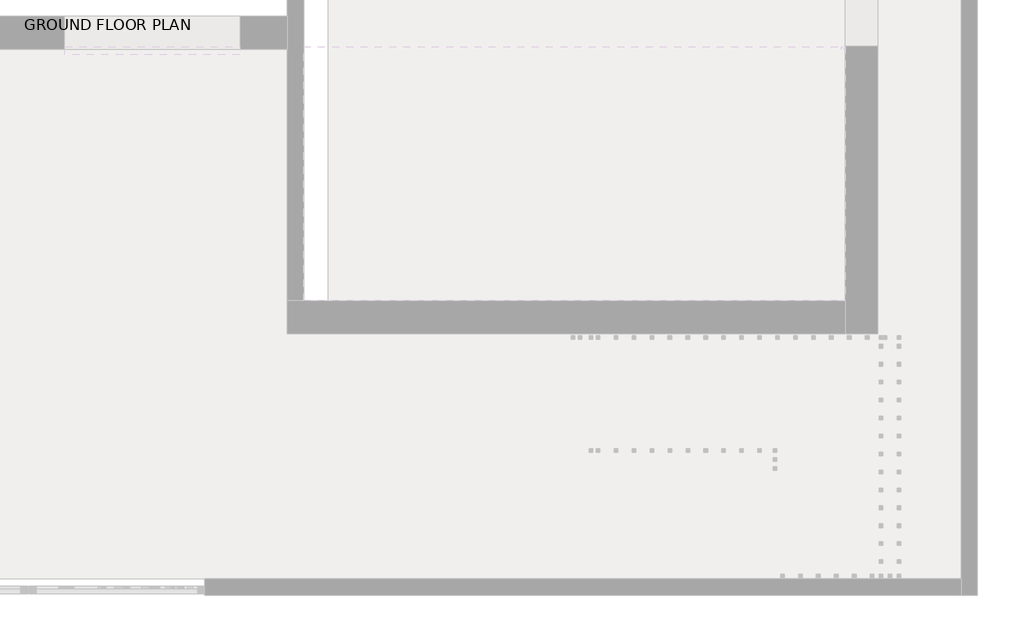
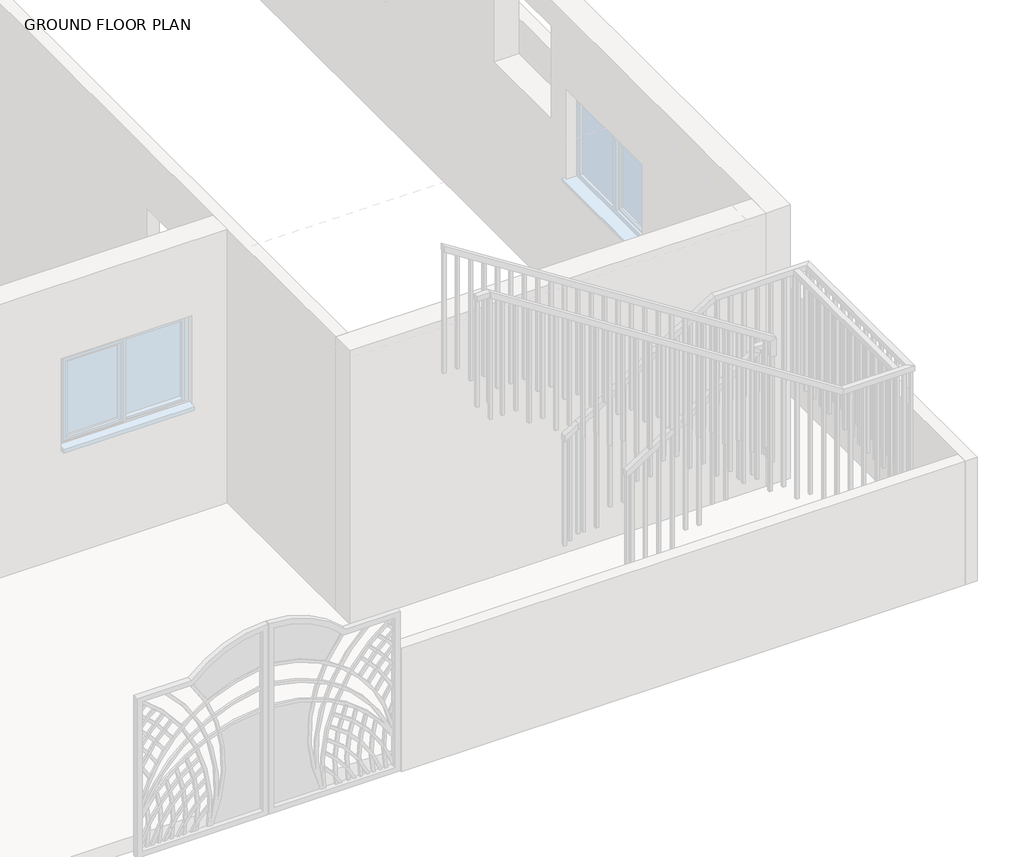
# One storey, part 19 of 23: 2 railings.
"""IFC4 building model written with IfcOpenShell, lengths in millimetres."""

from ifc_helpers import new_model, si_unit, frame, origin, place, context, project, spatial, polyline, outline, extrude, faceted_brep, element, save

model = new_model("IFC4")

# Units and contexts
model_context = context("Model", 3, world=origin())
ifc_project = project(units=[si_unit("LENGTHUNIT", "METRE", prefix="MILLI")], contexts=[model_context])

# Site, building, storey
site = spatial("IfcSite", under=ifc_project)
building = spatial("IfcBuilding", under=site)
storey = spatial("IfcBuildingStorey", under=building, Name="GROUND FLOOR PLAN", Elevation=487.68)

# Railings
placement = place(None, origin())
element("IfcRailing", 1, ObjectType="1100mm", at=placement, inside=storey, context=model_context, shape_type="SolidModel", body=[
    faceted_brep([(-8680.149573, -10220.0521308, 1912.8), (-8680.149573, -10220.0521308, 1853.4423995), (-8680.149573, -10270.0521308, 1853.4423995), (-8680.149573, -10270.0521308, 1912.8), (-7409.7306254, -10220.0521308, 2725.6), (-7395.1045513, -10220.0521308, 2675.6), (-7395.1045513, -10270.0521308, 2675.6), (-7409.7306254, -10270.0521308, 2725.6), (-6495.8132565, -10220.0521308, 2725.6), (-6495.8132565, -10220.0521308, 2675.6), (-6545.8132565, -10270.0521308, 2675.6), (-6545.8132565, -10270.0521308, 2725.6), (-6495.8132565, -11933.6860066, 2725.6), (-6495.8132565, -11933.6860066, 2675.6), (-6545.8132565, -11883.6860066, 2675.6), (-6545.8132565, -11883.6860066, 2725.6), (-7155.718398, -11933.6860066, 2725.6), (-7170.3479429, -11933.6860066, 2675.6), (-7170.3479429, -11883.6860066, 2675.6), (-7155.718398, -11883.6860066, 2725.6), (-10457.8773536, -11933.6860066, 4838.88), (-10457.8773536, -11883.6860066, 4838.88), (-10457.8773536, -11883.6860066, 4779.517542), (-10457.8773536, -11933.6860066, 4779.517542)], [[[0, 1, 2, 3]], [[1, 0, 4, 5]], [[2, 1, 5, 6]], [[3, 2, 6, 7]], [[0, 3, 7, 4]], [[5, 4, 8, 9]], [[6, 5, 9, 10]], [[7, 6, 10, 11]], [[4, 7, 11, 8]], [[9, 8, 12, 13]], [[10, 9, 13, 14]], [[11, 10, 14, 15]], [[8, 11, 15, 12]], [[13, 12, 16, 17]], [[14, 13, 17, 18]], [[15, 14, 18, 19]], [[12, 15, 19, 16]], [[20, 21, 22, 23]], [[17, 16, 20, 23]], [[18, 17, 23, 22]], [[19, 18, 22, 21]], [[16, 19, 21, 20]]]),
    extrude(outline(polyline([(4691.8007425, -10320.8132565), (4707.7999723, -10345.8132565), (3576.32, -10345.8132565), (3576.32, -10320.8132565), (4691.8007425, -10320.8132565)])), frame((0.0, -11921.1860066, 0.0), z_axis=(0.0, 1.0, 0.0), x_axis=(0.0, 0.0, 1.0)), (0.0, 0.0, 1.0), 25.0),
    extrude(outline(polyline([(4611.8045935, -10195.8132565), (4627.8038233, -10220.8132565), (3576.32, -10220.8132565), (3576.32, -10195.8132565), (4611.8045935, -10195.8132565)])), frame((0.0, -11921.1860066, 0.0), z_axis=(0.0, 1.0, 0.0), x_axis=(0.0, 0.0, 1.0)), (0.0, 0.0, 1.0), 25.0),
    extrude(outline(polyline([(4531.8084444, -10070.8132565), (4547.8076742, -10095.8132565), (3413.76, -10095.8132565), (3413.76, -10070.8132565), (4531.8084444, -10070.8132565)])), frame((0.0, -11921.1860066, 0.0), z_axis=(0.0, 1.0, 0.0), x_axis=(0.0, 0.0, 1.0)), (0.0, 0.0, 1.0), 25.0),
    extrude(outline(polyline([(4451.8122954, -9945.8132565), (4467.8115252, -9970.8132565), (3413.76, -9970.8132565), (3413.76, -9945.8132565), (4451.8122954, -9945.8132565)])), frame((0.0, -11921.1860066, 0.0), z_axis=(0.0, 1.0, 0.0), x_axis=(0.0, 0.0, 1.0)), (0.0, 0.0, 1.0), 25.0),
    extrude(outline(polyline([(4371.8161463, -9820.8132565), (4387.8153761, -9845.8132565), (3251.2, -9845.8132565), (3251.2, -9820.8132565), (4371.8161463, -9820.8132565)])), frame((0.0, -11921.1860066, 0.0), z_axis=(0.0, 1.0, 0.0), x_axis=(0.0, 0.0, 1.0)), (0.0, 0.0, 1.0), 25.0),
    extrude(outline(polyline([(4291.8423995, -9695.8132565), (4307.8371231, -9720.8132565), (3251.2, -9720.8132565), (3251.2, -9695.8132565), (4291.8423995, -9695.8132565)])), frame((0.0, -11921.1860066, 0.0), z_axis=(0.0, 1.0, 0.0), x_axis=(0.0, 0.0, 1.0)), (0.0, 0.0, 1.0), 25.0),
    extrude(outline(polyline([(4211.8238482, -9570.8132565), (4227.823078, -9595.8132565), (3088.64, -9595.8132565), (3088.64, -9570.8132565), (4211.8238482, -9570.8132565)])), frame((0.0, -11921.1860066, 0.0), z_axis=(0.0, 1.0, 0.0), x_axis=(0.0, 0.0, 1.0)), (0.0, 0.0, 1.0), 25.0),
    extrude(outline(polyline([(4131.8276992, -9445.8132565), (4147.826929, -9470.8132565), (3088.64, -9470.8132565), (3088.64, -9445.8132565), (4131.8276992, -9445.8132565)])), frame((0.0, -11921.1860066, 0.0), z_axis=(0.0, 1.0, 0.0), x_axis=(0.0, 0.0, 1.0)), (0.0, 0.0, 1.0), 25.0),
    extrude(outline(polyline([(4051.8315501, -9320.8132565), (4067.8307799, -9345.8132565), (2926.08, -9345.8132565), (2926.08, -9320.8132565), (4051.8315501, -9320.8132565)])), frame((0.0, -11921.1860066, 0.0), z_axis=(0.0, 1.0, 0.0), x_axis=(0.0, 0.0, 1.0)), (0.0, 0.0, 1.0), 25.0),
    extrude(outline(polyline([(3971.835401, -9195.8132565), (3987.8346309, -9220.8132565), (2926.08, -9220.8132565), (2926.08, -9195.8132565), (3971.835401, -9195.8132565)])), frame((0.0, -11921.1860066, 0.0), z_axis=(0.0, 1.0, 0.0), x_axis=(0.0, 0.0, 1.0)), (0.0, 0.0, 1.0), 25.0),
    extrude(outline(polyline([(3891.839252, -9070.8132565), (3907.8384818, -9095.8132565), (2763.52, -9095.8132565), (2763.52, -9070.8132565), (3891.839252, -9070.8132565)])), frame((0.0, -11921.1860066, 0.0), z_axis=(0.0, 1.0, 0.0), x_axis=(0.0, 0.0, 1.0)), (0.0, 0.0, 1.0), 25.0),
    extrude(outline(polyline([(3811.8431029, -8945.8132565), (3827.8423328, -8970.8132565), (2763.52, -8970.8132565), (2763.52, -8945.8132565), (3811.8431029, -8945.8132565)])), frame((0.0, -11921.1860066, 0.0), z_axis=(0.0, 1.0, 0.0), x_axis=(0.0, 0.0, 1.0)), (0.0, 0.0, 1.0), 25.0),
    extrude(outline(polyline([(3731.8469539, -8820.8132565), (3747.8461837, -8845.8132565), (2600.96, -8845.8132565), (2600.96, -8820.8132565), (3731.8469539, -8820.8132565)])), frame((0.0, -11921.1860066, 0.0), z_axis=(0.0, 1.0, 0.0), x_axis=(0.0, 0.0, 1.0)), (0.0, 0.0, 1.0), 25.0),
    extrude(outline(polyline([(3651.8508048, -8695.8132565), (3667.8500347, -8720.8132565), (2600.96, -8720.8132565), (2600.96, -8695.8132565), (3651.8508048, -8695.8132565)])), frame((0.0, -11921.1860066, 0.0), z_axis=(0.0, 1.0, 0.0), x_axis=(0.0, 0.0, 1.0)), (0.0, 0.0, 1.0), 25.0),
    extrude(outline(polyline([(3571.8546558, -8570.8132565), (3587.8538856, -8595.8132565), (2438.4, -8595.8132565), (2438.4, -8570.8132565), (3571.8546558, -8570.8132565)])), frame((0.0, -11921.1860066, 0.0), z_axis=(0.0, 1.0, 0.0), x_axis=(0.0, 0.0, 1.0)), (0.0, 0.0, 1.0), 25.0),
    extrude(outline(polyline([(3491.8585067, -8445.8132565), (3507.8577365, -8470.8132565), (2438.4, -8470.8132565), (2438.4, -8445.8132565), (3491.8585067, -8445.8132565)])), frame((0.0, -11921.1860066, 0.0), z_axis=(0.0, 1.0, 0.0), x_axis=(0.0, 0.0, 1.0)), (0.0, 0.0, 1.0), 25.0),
    extrude(outline(polyline([(3411.8623577, -8320.8132565), (3427.8615875, -8345.8132565), (2275.84, -8345.8132565), (2275.84, -8320.8132565), (3411.8623577, -8320.8132565)])), frame((0.0, -11921.1860066, 0.0), z_axis=(0.0, 1.0, 0.0), x_axis=(0.0, 0.0, 1.0)), (0.0, 0.0, 1.0), 25.0),
    extrude(outline(polyline([(3331.8662086, -8195.8132565), (3347.8654384, -8220.8132565), (2275.84, -8220.8132565), (2275.84, -8195.8132565), (3331.8662086, -8195.8132565)])), frame((0.0, -11921.1860066, 0.0), z_axis=(0.0, 1.0, 0.0), x_axis=(0.0, 0.0, 1.0)), (0.0, 0.0, 1.0), 25.0),
    extrude(outline(polyline([(3251.8700596, -8070.8132565), (3267.8692894, -8095.8132565), (2113.28, -8095.8132565), (2113.28, -8070.8132565), (3251.8700596, -8070.8132565)])), frame((0.0, -11921.1860066, 0.0), z_axis=(0.0, 1.0, 0.0), x_axis=(0.0, 0.0, 1.0)), (0.0, 0.0, 1.0), 25.0),
    extrude(outline(polyline([(3171.8739105, -7945.8132565), (3187.8731403, -7970.8132565), (2113.28, -7970.8132565), (2113.28, -7945.8132565), (3171.8739105, -7945.8132565)])), frame((0.0, -11921.1860066, 0.0), z_axis=(0.0, 1.0, 0.0), x_axis=(0.0, 0.0, 1.0)), (0.0, 0.0, 1.0), 25.0),
    extrude(outline(polyline([(3091.8777615, -7820.8132565), (3107.8769913, -7845.8132565), (1950.72, -7845.8132565), (1950.72, -7820.8132565), (3091.8777615, -7820.8132565)])), frame((0.0, -11921.1860066, 0.0), z_axis=(0.0, 1.0, 0.0), x_axis=(0.0, 0.0, 1.0)), (0.0, 0.0, 1.0), 25.0),
    extrude(outline(polyline([(3011.8816124, -7695.8132565), (3027.8808422, -7720.8132565), (1950.72, -7720.8132565), (1950.72, -7695.8132565), (3011.8816124, -7695.8132565)])), frame((0.0, -11921.1860066, 0.0), z_axis=(0.0, 1.0, 0.0), x_axis=(0.0, 0.0, 1.0)), (0.0, 0.0, 1.0), 25.0),
    extrude(outline(polyline([(2931.8854634, -7570.8132565), (2947.8846932, -7595.8132565), (1788.16, -7595.8132565), (1788.16, -7570.8132565), (2931.8854634, -7570.8132565)])), frame((0.0, -11921.1860066, 0.0), z_axis=(0.0, 1.0, 0.0), x_axis=(0.0, 0.0, 1.0)), (0.0, 0.0, 1.0), 25.0),
    extrude(outline(polyline([(2851.8893143, -7445.8132565), (2867.8885441, -7470.8132565), (1788.16, -7470.8132565), (1788.16, -7445.8132565), (2851.8893143, -7445.8132565)])), frame((0.0, -11921.1860066, 0.0), z_axis=(0.0, 1.0, 0.0), x_axis=(0.0, 0.0, 1.0)), (0.0, 0.0, 1.0), 25.0),
    extrude(outline(polyline([(2771.8931653, -7320.8132565), (2787.8923951, -7345.8132565), (1625.6, -7345.8132565), (1625.6, -7320.8132565), (2771.8931653, -7320.8132565)])), frame((0.0, -11921.1860066, 0.0), z_axis=(0.0, 1.0, 0.0), x_axis=(0.0, 0.0, 1.0)), (0.0, 0.0, 1.0), 25.0),
    extrude(outline(polyline([(2691.8970162, -7195.8132565), (2707.896246, -7220.8132565), (1625.6, -7220.8132565), (1625.6, -7195.8132565), (2691.8970162, -7195.8132565)])), frame((0.0, -11921.1860066, 0.0), z_axis=(0.0, 1.0, 0.0), x_axis=(0.0, 0.0, 1.0)), (0.0, 0.0, 1.0), 25.0),
    extrude(outline(polyline([(-7070.8132565, -11921.1860066), (-7095.8132565, -11921.1860066), (-7095.8132565, -11896.1860066), (-7070.8132565, -11896.1860066), (-7070.8132565, -11921.1860066)])), frame((0.0, 0.0, 1625.6), z_axis=(0.0, 0.0, 1.0), x_axis=(1.0, 0.0, 0.0)), (0.0, 0.0, 1.0), 1050.0),
    extrude(outline(polyline([(-6945.8132565, -11921.1860066), (-6970.8132565, -11921.1860066), (-6970.8132565, -11896.1860066), (-6945.8132565, -11896.1860066), (-6945.8132565, -11921.1860066)])), frame((0.0, 0.0, 1625.6), z_axis=(0.0, 0.0, 1.0), x_axis=(1.0, 0.0, 0.0)), (0.0, 0.0, 1.0), 1050.0),
    extrude(outline(polyline([(-6820.8132565, -11921.1860066), (-6845.8132565, -11921.1860066), (-6845.8132565, -11896.1860066), (-6820.8132565, -11896.1860066), (-6820.8132565, -11921.1860066)])), frame((0.0, 0.0, 1625.6), z_axis=(0.0, 0.0, 1.0), x_axis=(1.0, 0.0, 0.0)), (0.0, 0.0, 1.0), 1050.0),
    extrude(outline(polyline([(-6695.8132565, -11921.1860066), (-6720.8132565, -11921.1860066), (-6720.8132565, -11896.1860066), (-6695.8132565, -11896.1860066), (-6695.8132565, -11921.1860066)])), frame((0.0, 0.0, 1625.6), z_axis=(0.0, 0.0, 1.0), x_axis=(1.0, 0.0, 0.0)), (0.0, 0.0, 1.0), 1050.0),
    extrude(outline(polyline([(-6570.8132565, -11921.1860066), (-6595.8132565, -11921.1860066), (-6595.8132565, -11896.1860066), (-6570.8132565, -11896.1860066), (-6570.8132565, -11921.1860066)])), frame((0.0, 0.0, 1625.6), z_axis=(0.0, 0.0, 1.0), x_axis=(1.0, 0.0, 0.0)), (0.0, 0.0, 1.0), 1050.0),
    extrude(outline(polyline([(-6508.3132565, -11795.0521308), (-6508.3132565, -11820.0521308), (-6533.3132565, -11820.0521308), (-6533.3132565, -11795.0521308), (-6508.3132565, -11795.0521308)])), frame((0.0, 0.0, 1625.6), z_axis=(0.0, 0.0, 1.0), x_axis=(1.0, 0.0, 0.0)), (0.0, 0.0, 1.0), 1050.0),
    extrude(outline(polyline([(-6508.3132565, -11670.0521308), (-6508.3132565, -11695.0521308), (-6533.3132565, -11695.0521308), (-6533.3132565, -11670.0521308), (-6508.3132565, -11670.0521308)])), frame((0.0, 0.0, 1625.6), z_axis=(0.0, 0.0, 1.0), x_axis=(1.0, 0.0, 0.0)), (0.0, 0.0, 1.0), 1050.0),
    extrude(outline(polyline([(-6508.3132565, -11545.0521308), (-6508.3132565, -11570.0521308), (-6533.3132565, -11570.0521308), (-6533.3132565, -11545.0521308), (-6508.3132565, -11545.0521308)])), frame((0.0, 0.0, 1625.6), z_axis=(0.0, 0.0, 1.0), x_axis=(1.0, 0.0, 0.0)), (0.0, 0.0, 1.0), 1050.0),
    extrude(outline(polyline([(-6508.3132565, -11420.0521308), (-6508.3132565, -11445.0521308), (-6533.3132565, -11445.0521308), (-6533.3132565, -11420.0521308), (-6508.3132565, -11420.0521308)])), frame((0.0, 0.0, 1625.6), z_axis=(0.0, 0.0, 1.0), x_axis=(1.0, 0.0, 0.0)), (0.0, 0.0, 1.0), 1050.0),
    extrude(outline(polyline([(-6508.3132565, -11295.0521308), (-6508.3132565, -11320.0521308), (-6533.3132565, -11320.0521308), (-6533.3132565, -11295.0521308), (-6508.3132565, -11295.0521308)])), frame((0.0, 0.0, 1625.6), z_axis=(0.0, 0.0, 1.0), x_axis=(1.0, 0.0, 0.0)), (0.0, 0.0, 1.0), 1050.0),
    extrude(outline(polyline([(-6508.3132565, -11170.0521308), (-6508.3132565, -11195.0521308), (-6533.3132565, -11195.0521308), (-6533.3132565, -11170.0521308), (-6508.3132565, -11170.0521308)])), frame((0.0, 0.0, 1625.6), z_axis=(0.0, 0.0, 1.0), x_axis=(1.0, 0.0, 0.0)), (0.0, 0.0, 1.0), 1050.0),
    extrude(outline(polyline([(-6508.3132565, -11045.0521308), (-6508.3132565, -11070.0521308), (-6533.3132565, -11070.0521308), (-6533.3132565, -11045.0521308), (-6508.3132565, -11045.0521308)])), frame((0.0, 0.0, 1625.6), z_axis=(0.0, 0.0, 1.0), x_axis=(1.0, 0.0, 0.0)), (0.0, 0.0, 1.0), 1050.0),
    extrude(outline(polyline([(-6508.3132565, -10920.0521308), (-6508.3132565, -10945.0521308), (-6533.3132565, -10945.0521308), (-6533.3132565, -10920.0521308), (-6508.3132565, -10920.0521308)])), frame((0.0, 0.0, 1625.6), z_axis=(0.0, 0.0, 1.0), x_axis=(1.0, 0.0, 0.0)), (0.0, 0.0, 1.0), 1050.0),
    extrude(outline(polyline([(-6508.3132565, -10795.0521308), (-6508.3132565, -10820.0521308), (-6533.3132565, -10820.0521308), (-6533.3132565, -10795.0521308), (-6508.3132565, -10795.0521308)])), frame((0.0, 0.0, 1625.6), z_axis=(0.0, 0.0, 1.0), x_axis=(1.0, 0.0, 0.0)), (0.0, 0.0, 1.0), 1050.0),
    extrude(outline(polyline([(-6508.3132565, -10670.0521308), (-6508.3132565, -10695.0521308), (-6533.3132565, -10695.0521308), (-6533.3132565, -10670.0521308), (-6508.3132565, -10670.0521308)])), frame((0.0, 0.0, 1625.6), z_axis=(0.0, 0.0, 1.0), x_axis=(1.0, 0.0, 0.0)), (0.0, 0.0, 1.0), 1050.0),
    extrude(outline(polyline([(-6508.3132565, -10545.0521308), (-6508.3132565, -10570.0521308), (-6533.3132565, -10570.0521308), (-6533.3132565, -10545.0521308), (-6508.3132565, -10545.0521308)])), frame((0.0, 0.0, 1625.6), z_axis=(0.0, 0.0, 1.0), x_axis=(1.0, 0.0, 0.0)), (0.0, 0.0, 1.0), 1050.0),
    extrude(outline(polyline([(-6508.3132565, -10420.0521308), (-6508.3132565, -10445.0521308), (-6533.3132565, -10445.0521308), (-6533.3132565, -10420.0521308), (-6508.3132565, -10420.0521308)])), frame((0.0, 0.0, 1625.6), z_axis=(0.0, 0.0, 1.0), x_axis=(1.0, 0.0, 0.0)), (0.0, 0.0, 1.0), 1050.0),
    extrude(outline(polyline([(-6508.3132565, -10295.0521308), (-6508.3132565, -10320.0521308), (-6533.3132565, -10320.0521308), (-6533.3132565, -10295.0521308), (-6508.3132565, -10295.0521308)])), frame((0.0, 0.0, 1625.6), z_axis=(0.0, 0.0, 1.0), x_axis=(1.0, 0.0, 0.0)), (0.0, 0.0, 1.0), 1050.0),
    extrude(outline(polyline([(-6630.149573, -10232.5521308), (-6605.149573, -10232.5521308), (-6605.149573, -10257.5521308), (-6630.149573, -10257.5521308), (-6630.149573, -10232.5521308)])), frame((0.0, 0.0, 1625.6), z_axis=(0.0, 0.0, 1.0), x_axis=(1.0, 0.0, 0.0)), (0.0, 0.0, 1.0), 1050.0),
    extrude(outline(polyline([(-6755.149573, -10232.5521308), (-6730.149573, -10232.5521308), (-6730.149573, -10257.5521308), (-6755.149573, -10257.5521308), (-6755.149573, -10232.5521308)])), frame((0.0, 0.0, 1625.6), z_axis=(0.0, 0.0, 1.0), x_axis=(1.0, 0.0, 0.0)), (0.0, 0.0, 1.0), 1050.0),
    extrude(outline(polyline([(-6880.149573, -10232.5521308), (-6855.149573, -10232.5521308), (-6855.149573, -10257.5521308), (-6880.149573, -10257.5521308), (-6880.149573, -10232.5521308)])), frame((0.0, 0.0, 1625.6), z_axis=(0.0, 0.0, 1.0), x_axis=(1.0, 0.0, 0.0)), (0.0, 0.0, 1.0), 1050.0),
    extrude(outline(polyline([(-7005.149573, -10232.5521308), (-6980.149573, -10232.5521308), (-6980.149573, -10257.5521308), (-7005.149573, -10257.5521308), (-7005.149573, -10232.5521308)])), frame((0.0, 0.0, 1625.6), z_axis=(0.0, 0.0, 1.0), x_axis=(1.0, 0.0, 0.0)), (0.0, 0.0, 1.0), 1050.0),
    extrude(outline(polyline([(-7130.149573, -10232.5521308), (-7105.149573, -10232.5521308), (-7105.149573, -10257.5521308), (-7130.149573, -10257.5521308), (-7130.149573, -10232.5521308)])), frame((0.0, 0.0, 1625.6), z_axis=(0.0, 0.0, 1.0), x_axis=(1.0, 0.0, 0.0)), (0.0, 0.0, 1.0), 1050.0),
    extrude(outline(polyline([(-7255.149573, -10232.5521308), (-7230.149573, -10232.5521308), (-7230.149573, -10257.5521308), (-7255.149573, -10257.5521308), (-7255.149573, -10232.5521308)])), frame((0.0, 0.0, 1625.6), z_axis=(0.0, 0.0, 1.0), x_axis=(1.0, 0.0, 0.0)), (0.0, 0.0, 1.0), 1050.0),
    extrude(outline(polyline([(-7380.149573, -10232.5521308), (-7355.149573, -10232.5521308), (-7355.149573, -10257.5521308), (-7380.149573, -10257.5521308), (-7380.149573, -10232.5521308)])), frame((0.0, 0.0, 1625.6), z_axis=(0.0, 0.0, 1.0), x_axis=(1.0, 0.0, 0.0)), (0.0, 0.0, 1.0), 1050.0),
    extrude(outline(polyline([(1463.04, -7505.149573), (1463.04, -7480.149573), (2621.1891352, -7480.149573), (2605.1944115, -7505.149573), (1463.04, -7505.149573)])), frame((0.0, -10257.5521308, 0.0), z_axis=(0.0, 1.0, 0.0), x_axis=(0.0, 0.0, 1.0)), (0.0, 0.0, 1.0), 25.0),
    extrude(outline(polyline([(1463.04, -7630.149573), (1463.04, -7605.149573), (2541.2155169, -7605.149573), (2525.2207932, -7630.149573), (1463.04, -7630.149573)])), frame((0.0, -10257.5521308, 0.0), z_axis=(0.0, 1.0, 0.0), x_axis=(0.0, 0.0, 1.0)), (0.0, 0.0, 1.0), 25.0),
    extrude(outline(polyline([(1300.48, -7755.149573), (1300.48, -7730.149573), (2461.2418986, -7730.149573), (2445.2471749, -7755.149573), (1300.48, -7755.149573)])), frame((0.0, -10257.5521308, 0.0), z_axis=(0.0, 1.0, 0.0), x_axis=(0.0, 0.0, 1.0)), (0.0, 0.0, 1.0), 25.0),
    extrude(outline(polyline([(1300.48, -7880.149573), (1300.48, -7855.149573), (2381.2682803, -7855.149573), (2365.2735566, -7880.149573), (1300.48, -7880.149573)])), frame((0.0, -10257.5521308, 0.0), z_axis=(0.0, 1.0, 0.0), x_axis=(0.0, 0.0, 1.0)), (0.0, 0.0, 1.0), 25.0),
    extrude(outline(polyline([(1137.92, -8005.149573), (1137.92, -7980.149573), (2301.294662, -7980.149573), (2285.2999383, -8005.149573), (1137.92, -8005.149573)])), frame((0.0, -10257.5521308, 0.0), z_axis=(0.0, 1.0, 0.0), x_axis=(0.0, 0.0, 1.0)), (0.0, 0.0, 1.0), 25.0),
    extrude(outline(polyline([(1137.92, -8130.149573), (1137.92, -8105.149573), (2221.3210437, -8105.149573), (2205.32632, -8130.149573), (1137.92, -8130.149573)])), frame((0.0, -10257.5521308, 0.0), z_axis=(0.0, 1.0, 0.0), x_axis=(0.0, 0.0, 1.0)), (0.0, 0.0, 1.0), 25.0),
    extrude(outline(polyline([(975.36, -8255.149573), (975.36, -8230.149573), (2141.3474254, -8230.149573), (2125.3527017, -8255.149573), (975.36, -8255.149573)])), frame((0.0, -10257.5521308, 0.0), z_axis=(0.0, 1.0, 0.0), x_axis=(0.0, 0.0, 1.0)), (0.0, 0.0, 1.0), 25.0),
    extrude(outline(polyline([(975.36, -8380.149573), (975.36, -8355.149573), (2061.3738071, -8355.149573), (2045.3790834, -8380.149573), (975.36, -8380.149573)])), frame((0.0, -10257.5521308, 0.0), z_axis=(0.0, 1.0, 0.0), x_axis=(0.0, 0.0, 1.0)), (0.0, 0.0, 1.0), 25.0),
    extrude(outline(polyline([(812.8, -8505.149573), (812.8, -8480.149573), (1981.4001888, -8480.149573), (1965.4054651, -8505.149573), (812.8, -8505.149573)])), frame((0.0, -10257.5521308, 0.0), z_axis=(0.0, 1.0, 0.0), x_axis=(0.0, 0.0, 1.0)), (0.0, 0.0, 1.0), 25.0),
    extrude(outline(polyline([(812.8, -8630.149573), (812.8, -8605.149573), (1901.4265705, -8605.149573), (1885.4318468, -8630.149573), (812.8, -8630.149573)])), frame((0.0, -10257.5521308, 0.0), z_axis=(0.0, 1.0, 0.0), x_axis=(0.0, 0.0, 1.0)), (0.0, 0.0, 1.0), 25.0),
    extrude(outline(polyline([(-6508.3132565, -11896.1860066), (-6508.3132565, -11921.1860066), (-6533.3132565, -11921.1860066), (-6533.3132565, -11896.1860066), (-6508.3132565, -11896.1860066)])), frame((0.0, 0.0, 1625.6), z_axis=(0.0, 0.0, 1.0), x_axis=(1.0, 0.0, 0.0)), (0.0, 0.0, 1.0), 1050.0),
    extrude(outline(polyline([(-6533.3132565, -10232.5521308), (-6508.3132565, -10232.5521308), (-6508.3132565, -10257.5521308), (-6533.3132565, -10257.5521308), (-6533.3132565, -10232.5521308)])), frame((0.0, 0.0, 1625.6), z_axis=(0.0, 0.0, 1.0), x_axis=(1.0, 0.0, 0.0)), (0.0, 0.0, 1.0), 1050.0),
    extrude(outline(polyline([(4763.5183122, -10432.8773536), (4779.517542, -10457.8773536), (3576.32, -10457.8773536), (3576.32, -10432.8773536), (4763.5183122, -10432.8773536)])), frame((0.0, -11921.1860066, 0.0), z_axis=(0.0, 1.0, 0.0), x_axis=(0.0, 0.0, 1.0)), (0.0, 0.0, 1.0), 25.0),
    extrude(outline(polyline([(812.8, -8680.149573), (812.8, -8655.149573), (1869.4371231, -8655.149573), (1853.4423995, -8680.149573), (812.8, -8680.149573)])), frame((0.0, -10257.5521308, 0.0), z_axis=(0.0, 1.0, 0.0), x_axis=(0.0, 0.0, 1.0)), (0.0, 0.0, 1.0), 25.0),
])
element("IfcRailing", 2, ObjectType="1100mm", at=placement, inside=storey, context=model_context, shape_type="SolidModel", body=[
    faceted_brep([(-8680.149573, -11007.9255223, 1912.8), (-8680.149573, -11007.9255223, 1853.4423995), (-8680.149573, -11057.9255223, 1853.4423995), (-8680.149573, -11057.9255223, 1912.8), (-7484.3306254, -11007.9255223, 2677.8717446), (-7434.3306254, -11007.9255223, 2650.5035914), (-7434.3306254, -11057.9255223, 2650.5035914), (-7484.3306254, -11057.9255223, 2677.8717446), (-7484.3306254, -11007.9255223, 2725.6), (-7434.3306254, -11007.9255223, 2675.6), (-7434.3306254, -11057.9255223, 2675.6), (-7484.3306254, -11057.9255223, 2725.6), (-7359.3306254, -11007.9255223, 2725.6), (-7359.3306254, -11007.9255223, 2675.6), (-7409.3306254, -11057.9255223, 2675.6), (-7409.3306254, -11057.9255223, 2725.6), (-7359.3306254, -11132.9255223, 2725.6), (-7359.3306254, -11132.9255223, 2675.6), (-7409.3306254, -11132.9255223, 2675.6), (-7409.3306254, -11132.9255223, 2725.6), (-7359.3306254, -11134.9255223, 2725.6), (-7409.3306254, -11134.9255223, 2725.6), (-7409.3306254, -11184.9255223, 2675.6), (-7359.3306254, -11184.9255223, 2675.6)], [[[0, 1, 2, 3]], [[1, 0, 4, 5]], [[2, 1, 5, 6]], [[3, 2, 6, 7]], [[0, 3, 7, 4]], [[5, 4, 8, 9]], [[6, 5, 9, 10]], [[7, 6, 10, 11]], [[4, 7, 11, 8]], [[9, 8, 12, 13]], [[10, 9, 13, 14]], [[11, 10, 14, 15]], [[8, 11, 15, 12]], [[13, 12, 16, 17]], [[14, 13, 17, 18]], [[15, 14, 18, 19]], [[12, 15, 19, 16]], [[20, 21, 22, 23]], [[17, 16, 20, 23]], [[18, 17, 23, 22]], [[19, 18, 22, 21]], [[16, 19, 21, 20]]]),
    faceted_brep([(-7359.3306254, -11184.9255223, 2855.9055527), (-7409.3306254, -11184.9255223, 2828.5415543), (-7409.3306254, -11134.9255223, 2828.5415543), (-7359.3306254, -11134.9255223, 2855.9055527), (-10457.8773536, -11184.9255223, 4838.88), (-10457.8773536, -11134.9255223, 4838.88), (-10457.8773536, -11134.9255223, 4779.517542), (-10457.8773536, -11184.9255223, 4779.517542)], [[[0, 1, 2, 3]], [[4, 5, 6, 7]], [[1, 0, 4, 7]], [[2, 1, 7, 6]], [[3, 2, 6, 5]], [[0, 3, 5, 4]]]),
    faceted_brep([(-7359.3306254, -11134.9255223, 2725.6), (-7359.3306254, -11184.9255223, 2675.6), (-7409.3306254, -11184.9255223, 2675.6), (-7409.3306254, -11134.9255223, 2725.6), (-7359.3306254, -11134.9255223, 2855.9055527), (-7409.3306254, -11134.9255223, 2828.5415543), (-7409.3306254, -11184.9255223, 2828.5415543), (-7359.3306254, -11184.9255223, 2855.9055527)], [[[0, 1, 2, 3]], [[4, 5, 6, 7]], [[1, 0, 4, 7]], [[2, 1, 7, 6]], [[3, 2, 6, 5]], [[0, 3, 5, 4]]]),
    extrude(outline(polyline([(3576.32, -10434.3306254), (4764.4483614, -10434.3306254), (4780.4475912, -10459.3306254), (3576.32, -10459.3306254), (3576.32, -10434.3306254)])), frame((0.0, -11172.4255223, 0.0), z_axis=(0.0, 1.0, 0.0), x_axis=(0.0, 0.0, 1.0)), (0.0, 0.0, 1.0), 25.0),
    extrude(outline(polyline([(3576.32, -10309.3306254), (4684.4522123, -10309.3306254), (4700.4514422, -10334.3306254), (3576.32, -10334.3306254), (3576.32, -10309.3306254)])), frame((0.0, -11172.4255223, 0.0), z_axis=(0.0, 1.0, 0.0), x_axis=(0.0, 0.0, 1.0)), (0.0, 0.0, 1.0), 25.0),
    extrude(outline(polyline([(3413.76, -10184.3306254), (4604.4560633, -10184.3306254), (4620.4552931, -10209.3306254), (3413.76, -10209.3306254), (3413.76, -10184.3306254)])), frame((0.0, -11172.4255223, 0.0), z_axis=(0.0, 1.0, 0.0), x_axis=(0.0, 0.0, 1.0)), (0.0, 0.0, 1.0), 25.0),
    extrude(outline(polyline([(3413.76, -10059.3306254), (4524.4599142, -10059.3306254), (4540.459144, -10084.3306254), (3413.76, -10084.3306254), (3413.76, -10059.3306254)])), frame((0.0, -11172.4255223, 0.0), z_axis=(0.0, 1.0, 0.0), x_axis=(0.0, 0.0, 1.0)), (0.0, 0.0, 1.0), 25.0),
    extrude(outline(polyline([(3251.2, -9934.3306254), (4444.4637652, -9934.3306254), (4460.462995, -9959.3306254), (3251.2, -9959.3306254), (3251.2, -9934.3306254)])), frame((0.0, -11172.4255223, 0.0), z_axis=(0.0, 1.0, 0.0), x_axis=(0.0, 0.0, 1.0)), (0.0, 0.0, 1.0), 25.0),
    extrude(outline(polyline([(3251.2, -9809.3306254), (4364.4676161, -9809.3306254), (4380.4668459, -9834.3306254), (3251.2, -9834.3306254), (3251.2, -9809.3306254)])), frame((0.0, -11172.4255223, 0.0), z_axis=(0.0, 1.0, 0.0), x_axis=(0.0, 0.0, 1.0)), (0.0, 0.0, 1.0), 25.0),
    extrude(outline(polyline([(3251.2, -9684.3306254), (4284.4714671, -9684.3306254), (4300.4706969, -9709.3306254), (3251.2, -9709.3306254), (3251.2, -9684.3306254)])), frame((0.0, -11172.4255223, 0.0), z_axis=(0.0, 1.0, 0.0), x_axis=(0.0, 0.0, 1.0)), (0.0, 0.0, 1.0), 25.0),
    extrude(outline(polyline([(3088.64, -9559.3306254), (4204.475318, -9559.3306254), (4220.4745478, -9584.3306254), (3088.64, -9584.3306254), (3088.64, -9559.3306254)])), frame((0.0, -11172.4255223, 0.0), z_axis=(0.0, 1.0, 0.0), x_axis=(0.0, 0.0, 1.0)), (0.0, 0.0, 1.0), 25.0),
    extrude(outline(polyline([(3088.64, -9434.3306254), (4124.479169, -9434.3306254), (4140.4783988, -9459.3306254), (3088.64, -9459.3306254), (3088.64, -9434.3306254)])), frame((0.0, -11172.4255223, 0.0), z_axis=(0.0, 1.0, 0.0), x_axis=(0.0, 0.0, 1.0)), (0.0, 0.0, 1.0), 25.0),
    extrude(outline(polyline([(2926.08, -9309.3306254), (4044.4830199, -9309.3306254), (4060.4822497, -9334.3306254), (2926.08, -9334.3306254), (2926.08, -9309.3306254)])), frame((0.0, -11172.4255223, 0.0), z_axis=(0.0, 1.0, 0.0), x_axis=(0.0, 0.0, 1.0)), (0.0, 0.0, 1.0), 25.0),
    extrude(outline(polyline([(2926.08, -9184.3306254), (3964.4868709, -9184.3306254), (3980.4861007, -9209.3306254), (2926.08, -9209.3306254), (2926.08, -9184.3306254)])), frame((0.0, -11172.4255223, 0.0), z_axis=(0.0, 1.0, 0.0), x_axis=(0.0, 0.0, 1.0)), (0.0, 0.0, 1.0), 25.0),
    extrude(outline(polyline([(2763.52, -9059.3306254), (3884.4907218, -9059.3306254), (3900.4899516, -9084.3306254), (2763.52, -9084.3306254), (2763.52, -9059.3306254)])), frame((0.0, -11172.4255223, 0.0), z_axis=(0.0, 1.0, 0.0), x_axis=(0.0, 0.0, 1.0)), (0.0, 0.0, 1.0), 25.0),
    extrude(outline(polyline([(2763.52, -8934.3306254), (3804.4945728, -8934.3306254), (3820.4938026, -8959.3306254), (2763.52, -8959.3306254), (2763.52, -8934.3306254)])), frame((0.0, -11172.4255223, 0.0), z_axis=(0.0, 1.0, 0.0), x_axis=(0.0, 0.0, 1.0)), (0.0, 0.0, 1.0), 25.0),
    extrude(outline(polyline([(2600.96, -8809.3306254), (3724.4984237, -8809.3306254), (3740.4976535, -8834.3306254), (2600.96, -8834.3306254), (2600.96, -8809.3306254)])), frame((0.0, -11172.4255223, 0.0), z_axis=(0.0, 1.0, 0.0), x_axis=(0.0, 0.0, 1.0)), (0.0, 0.0, 1.0), 25.0),
    extrude(outline(polyline([(2600.96, -8684.3306254), (3644.5022747, -8684.3306254), (3660.5015045, -8709.3306254), (2600.96, -8709.3306254), (2600.96, -8684.3306254)])), frame((0.0, -11172.4255223, 0.0), z_axis=(0.0, 1.0, 0.0), x_axis=(0.0, 0.0, 1.0)), (0.0, 0.0, 1.0), 25.0),
    extrude(outline(polyline([(2438.4, -8559.3306254), (3564.5061256, -8559.3306254), (3580.5053554, -8584.3306254), (2438.4, -8584.3306254), (2438.4, -8559.3306254)])), frame((0.0, -11172.4255223, 0.0), z_axis=(0.0, 1.0, 0.0), x_axis=(0.0, 0.0, 1.0)), (0.0, 0.0, 1.0), 25.0),
    extrude(outline(polyline([(2438.4, -8434.3306254), (3484.5099766, -8434.3306254), (3500.5092064, -8459.3306254), (2438.4, -8459.3306254), (2438.4, -8434.3306254)])), frame((0.0, -11172.4255223, 0.0), z_axis=(0.0, 1.0, 0.0), x_axis=(0.0, 0.0, 1.0)), (0.0, 0.0, 1.0), 25.0),
    extrude(outline(polyline([(2275.84, -8309.3306254), (3404.5138275, -8309.3306254), (3420.5130573, -8334.3306254), (2275.84, -8334.3306254), (2275.84, -8309.3306254)])), frame((0.0, -11172.4255223, 0.0), z_axis=(0.0, 1.0, 0.0), x_axis=(0.0, 0.0, 1.0)), (0.0, 0.0, 1.0), 25.0),
    extrude(outline(polyline([(2275.84, -8184.3306254), (3324.5176785, -8184.3306254), (3340.5169083, -8209.3306254), (2275.84, -8209.3306254), (2275.84, -8184.3306254)])), frame((0.0, -11172.4255223, 0.0), z_axis=(0.0, 1.0, 0.0), x_axis=(0.0, 0.0, 1.0)), (0.0, 0.0, 1.0), 25.0),
    extrude(outline(polyline([(2113.28, -8059.3306254), (3244.5215294, -8059.3306254), (3260.5207592, -8084.3306254), (2113.28, -8084.3306254), (2113.28, -8059.3306254)])), frame((0.0, -11172.4255223, 0.0), z_axis=(0.0, 1.0, 0.0), x_axis=(0.0, 0.0, 1.0)), (0.0, 0.0, 1.0), 25.0),
    extrude(outline(polyline([(2113.28, -7934.3306254), (3164.5253804, -7934.3306254), (3180.5246102, -7959.3306254), (2113.28, -7959.3306254), (2113.28, -7934.3306254)])), frame((0.0, -11172.4255223, 0.0), z_axis=(0.0, 1.0, 0.0), x_axis=(0.0, 0.0, 1.0)), (0.0, 0.0, 1.0), 25.0),
    extrude(outline(polyline([(1950.72, -7809.3306254), (3084.5292313, -7809.3306254), (3100.5284611, -7834.3306254), (1950.72, -7834.3306254), (1950.72, -7809.3306254)])), frame((0.0, -11172.4255223, 0.0), z_axis=(0.0, 1.0, 0.0), x_axis=(0.0, 0.0, 1.0)), (0.0, 0.0, 1.0), 25.0),
    extrude(outline(polyline([(1950.72, -7684.3306254), (3004.5330823, -7684.3306254), (3020.5323121, -7709.3306254), (1950.72, -7709.3306254), (1950.72, -7684.3306254)])), frame((0.0, -11172.4255223, 0.0), z_axis=(0.0, 1.0, 0.0), x_axis=(0.0, 0.0, 1.0)), (0.0, 0.0, 1.0), 25.0),
    extrude(outline(polyline([(1788.16, -7559.3306254), (2924.5369332, -7559.3306254), (2940.536163, -7584.3306254), (1788.16, -7584.3306254), (1788.16, -7559.3306254)])), frame((0.0, -11172.4255223, 0.0), z_axis=(0.0, 1.0, 0.0), x_axis=(0.0, 0.0, 1.0)), (0.0, 0.0, 1.0), 25.0),
    extrude(outline(polyline([(1788.16, -7434.3306254), (2844.5407841, -7434.3306254), (2860.540014, -7459.3306254), (1788.16, -7459.3306254), (1788.16, -7434.3306254)])), frame((0.0, -11172.4255223, 0.0), z_axis=(0.0, 1.0, 0.0), x_axis=(0.0, 0.0, 1.0)), (0.0, 0.0, 1.0), 25.0),
    extrude(outline(polyline([(-7396.8306254, -11082.9255223), (-7371.8306254, -11082.9255223), (-7371.8306254, -11107.9255223), (-7396.8306254, -11107.9255223), (-7396.8306254, -11082.9255223)])), frame((0.0, 0.0, 1625.6), z_axis=(0.0, 0.0, 1.0), x_axis=(1.0, 0.0, 0.0)), (0.0, 0.0, 1.0), 1050.0),
    extrude(outline(polyline([(2605.1944115, -7505.149573), (1463.04, -7505.149573), (1463.04, -7480.149573), (2621.1891352, -7480.149573), (2605.1944115, -7505.149573)])), frame((0.0, -11045.4255223, 0.0), z_axis=(0.0, 1.0, 0.0), x_axis=(0.0, 0.0, 1.0)), (0.0, 0.0, 1.0), 25.0),
    extrude(outline(polyline([(2525.2207932, -7630.149573), (1463.04, -7630.149573), (1463.04, -7605.149573), (2541.2155169, -7605.149573), (2525.2207932, -7630.149573)])), frame((0.0, -11045.4255223, 0.0), z_axis=(0.0, 1.0, 0.0), x_axis=(0.0, 0.0, 1.0)), (0.0, 0.0, 1.0), 25.0),
    extrude(outline(polyline([(2445.2471749, -7755.149573), (1300.48, -7755.149573), (1300.48, -7730.149573), (2461.2418986, -7730.149573), (2445.2471749, -7755.149573)])), frame((0.0, -11045.4255223, 0.0), z_axis=(0.0, 1.0, 0.0), x_axis=(0.0, 0.0, 1.0)), (0.0, 0.0, 1.0), 25.0),
    extrude(outline(polyline([(2365.2735566, -7880.149573), (1300.48, -7880.149573), (1300.48, -7855.149573), (2381.2682803, -7855.149573), (2365.2735566, -7880.149573)])), frame((0.0, -11045.4255223, 0.0), z_axis=(0.0, 1.0, 0.0), x_axis=(0.0, 0.0, 1.0)), (0.0, 0.0, 1.0), 25.0),
    extrude(outline(polyline([(2285.2999383, -8005.149573), (1137.92, -8005.149573), (1137.92, -7980.149573), (2301.294662, -7980.149573), (2285.2999383, -8005.149573)])), frame((0.0, -11045.4255223, 0.0), z_axis=(0.0, 1.0, 0.0), x_axis=(0.0, 0.0, 1.0)), (0.0, 0.0, 1.0), 25.0),
    extrude(outline(polyline([(2205.32632, -8130.149573), (1137.92, -8130.149573), (1137.92, -8105.149573), (2221.3210437, -8105.149573), (2205.32632, -8130.149573)])), frame((0.0, -11045.4255223, 0.0), z_axis=(0.0, 1.0, 0.0), x_axis=(0.0, 0.0, 1.0)), (0.0, 0.0, 1.0), 25.0),
    extrude(outline(polyline([(2125.3527017, -8255.149573), (975.36, -8255.149573), (975.36, -8230.149573), (2141.3474254, -8230.149573), (2125.3527017, -8255.149573)])), frame((0.0, -11045.4255223, 0.0), z_axis=(0.0, 1.0, 0.0), x_axis=(0.0, 0.0, 1.0)), (0.0, 0.0, 1.0), 25.0),
    extrude(outline(polyline([(2045.3790834, -8380.149573), (975.36, -8380.149573), (975.36, -8355.149573), (2061.3738071, -8355.149573), (2045.3790834, -8380.149573)])), frame((0.0, -11045.4255223, 0.0), z_axis=(0.0, 1.0, 0.0), x_axis=(0.0, 0.0, 1.0)), (0.0, 0.0, 1.0), 25.0),
    extrude(outline(polyline([(1965.4054651, -8505.149573), (812.8, -8505.149573), (812.8, -8480.149573), (1981.4001888, -8480.149573), (1965.4054651, -8505.149573)])), frame((0.0, -11045.4255223, 0.0), z_axis=(0.0, 1.0, 0.0), x_axis=(0.0, 0.0, 1.0)), (0.0, 0.0, 1.0), 25.0),
    extrude(outline(polyline([(1885.4318468, -8630.149573), (812.8, -8630.149573), (812.8, -8605.149573), (1901.4265705, -8605.149573), (1885.4318468, -8630.149573)])), frame((0.0, -11045.4255223, 0.0), z_axis=(0.0, 1.0, 0.0), x_axis=(0.0, 0.0, 1.0)), (0.0, 0.0, 1.0), 25.0),
    extrude(outline(polyline([(-7396.8306254, -11147.4255223), (-7371.8306254, -11147.4255223), (-7371.8306254, -11172.4255223), (-7396.8306254, -11172.4255223), (-7396.8306254, -11147.4255223)])), frame((0.0, 0.0, 1625.6), z_axis=(0.0, 0.0, 1.0), x_axis=(1.0, 0.0, 0.0)), (0.0, 0.0, 1.0), 1050.0),
    extrude(outline(polyline([(-7396.8306254, -11045.4255223), (-7396.8306254, -11020.4255223), (-7371.8306254, -11020.4255223), (-7371.8306254, -11045.4255223), (-7396.8306254, -11045.4255223)])), frame((0.0, 0.0, 1625.6), z_axis=(0.0, 0.0, 1.0), x_axis=(1.0, 0.0, 0.0)), (0.0, 0.0, 1.0), 1050.0),
    extrude(outline(polyline([(3576.32, -10432.8773536), (4763.5183122, -10432.8773536), (4779.517542, -10457.8773536), (3576.32, -10457.8773536), (3576.32, -10432.8773536)])), frame((0.0, -11172.4255223, 0.0), z_axis=(0.0, 1.0, 0.0), x_axis=(0.0, 0.0, 1.0)), (0.0, 0.0, 1.0), 25.0),
    extrude(outline(polyline([(1853.4423995, -8680.149573), (812.8, -8680.149573), (812.8, -8655.149573), (1869.4371231, -8655.149573), (1853.4423995, -8680.149573)])), frame((0.0, -11045.4255223, 0.0), z_axis=(0.0, 1.0, 0.0), x_axis=(0.0, 0.0, 1.0)), (0.0, 0.0, 1.0), 25.0),
])

save(model, "model.ifc")

# Revit data of these elements
# Type "1100mm"
#   built-in parameter 1008612 = 0.019685 (stored number, unit not read)
#   built-in parameter 1008611 = 0.019685 (stored number, unit not read)
#   built-in parameter 1008609 = 0.902231 (stored number, unit not read)
#   built-in parameter 1008604 = 0.19685 (stored number, unit not read)
#   built-in parameter 1008603 = 0.164042 (stored number, unit not read)
#   Railing Height = 3.608924 ft
#   built-in parameter 1008630 = 2
#   built-in parameter 1008610 = 2
#   built-in parameter 1008608 = 1
#   built-in parameter 1008618 = Baluster_Square : 25mm
# Elements 1, 2 (IfcRailing, "1100mm")
#   Phase Created = New Construction
